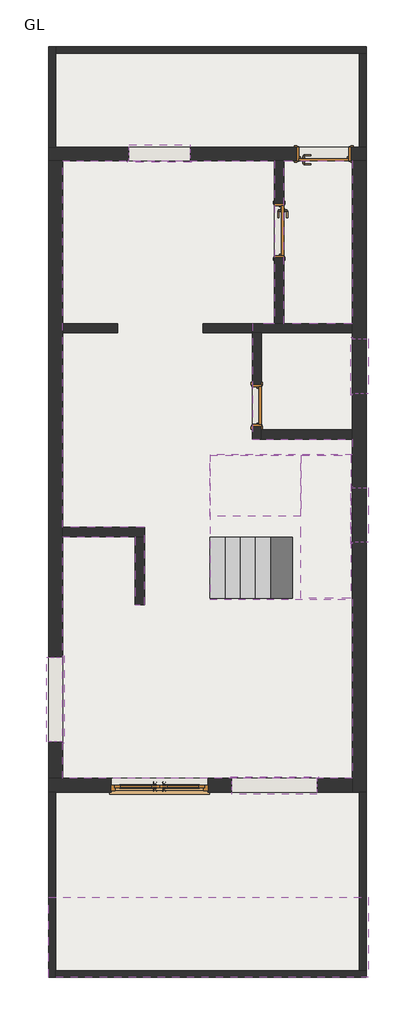
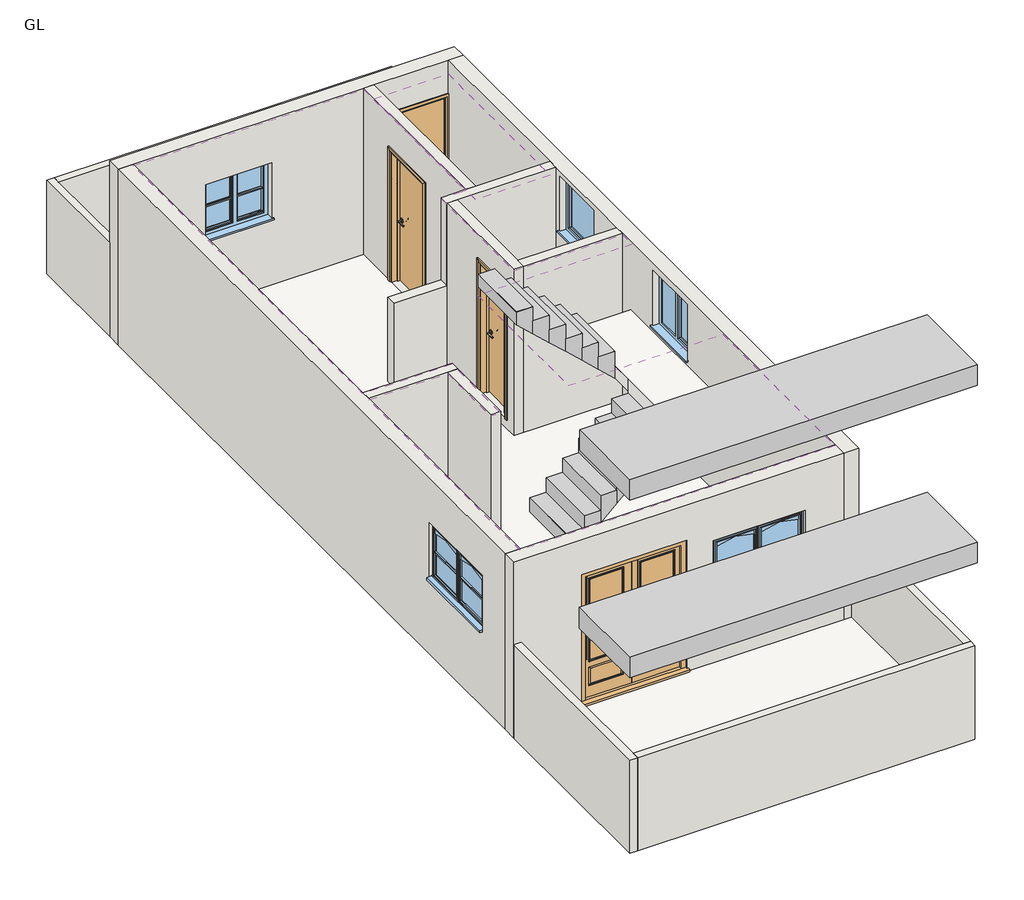
# One storey, incomplete: 18 walls, 6 slabs, 5 windows, 4 doors, 2 coverings, 2 stair flights, 1 furniture element.
"""IFC4 building model written with IfcOpenShell, lengths in millimetres."""

from ifc_helpers import new_model, si_unit, frame, origin, origin_with_axes, place, context, project, spatial, polyline, outline, extrude, faceted_brep, transform, mapped, element, save
from components import doors_extdbl_w_glazing_bars_2_f0b4ebcb, doors_extdbl_w_glazing_bars_2_fbc7e696, doors_intsgl_1_0_7m_00cad461, doors_intsgl_1_0_9m_9bbf83a0, doors_intsgl_1_0_9m_7aac3a70, casework_2_casework_2_475e0740, windows_dbl_swept_head_1_m_37dff1ae, windows_dbl_swept_head_1_4_m_8667dff2, windows_dbl_variable_casement_3235f540, windows_sgl_plain_0_9_m_ad1c2cf7

model = new_model("IFC4")

# Units and contexts
model_context = context("Model", 3, world=origin())
ifc_project = project(units=[si_unit("LENGTHUNIT", "METRE", prefix="MILLI")], contexts=[model_context])

# Site, building, storey
site = spatial("IfcSite", under=ifc_project)
building = spatial("IfcBuilding", under=site)
storey = spatial("IfcBuildingStorey", under=building, Name="GL", Elevation=0.0)

# Coverings
placement = place(None, origin())
element("IfcCovering", 1, ObjectType="Plain", at=placement, inside=storey, context=model_context, shape_type="SweptSolid", body=[
    extrude(outline(polyline([(-17484.6794706, 12010.5758404), (-16354.2794706, 12010.5758404), (-16354.2794706, 9327.0908033), (-17484.6794706, 9327.0908033), (-17484.6794706, 12010.5758404)])), frame((0.0, 0.0, 2600.0), z_axis=(0.0, 0.0, 1.0), x_axis=(1.0, 0.0, 0.0)), (0.0, 0.0, 1.0), 57.0),
])
element("IfcCovering", 2, ObjectType="Plain", at=placement, inside=storey, context=model_context, shape_type="SweptSolid", body=[
    extrude(outline(polyline([(-21137.0794706, 12010.5758404), (-17637.0794706, 12010.5758404), (-17637.0794706, 9327.0908033), (-18006.6794706, 9327.0908033), (-18006.6794706, 7422.2908033), (-16354.2794706, 7422.2908033), (-16354.2794706, 7168.7350753), (-18701.8794706, 7168.7350753), (-18701.8794706, 4785.9166056), (-16354.2794706, 4785.9166056), (-16354.2794706, 1829.2258404), (-21137.0794706, 1829.2258404), (-21137.0794706, 5814.1913528), (-19937.0794706, 5814.1913528), (-19937.0794706, 4690.3913528), (-19784.6794706, 4690.3913528), (-19784.6794706, 5966.5913528), (-21137.0794706, 5966.5913528), (-21137.0794706, 12010.5758404)])), frame((0.0, 0.0, 2800.0), z_axis=(0.0, 0.0, 1.0), x_axis=(1.0, 0.0, 0.0)), (0.0, 0.0, 1.0), 57.0),
])

# Doors
doors_extdbl_w_glazing_bars_2_shape = doors_extdbl_w_glazing_bars_2_f0b4ebcb(model_context)
doors_extdbl_w_glazing_bars_2_2_shape = doors_extdbl_w_glazing_bars_2_fbc7e696(model_context)
element("IfcDoor", 3, ObjectType="Doors_ExtDbl_w-Glazing_Bars_2", at=placement, inside=storey, context=model_context, shape_type="MappedRepresentation", body=[
    mapped(doors_extdbl_w_glazing_bars_2_shape, transform((-19537.0794706, 1714.9258404, 150.0), x_axis=(-1.0, 0.0, 0.0), y_axis=(0.0, -1.0, 0.0), z_axis=(0.0, 0.0, 1.0))),
    mapped(doors_extdbl_w_glazing_bars_2_2_shape, transform((-19537.0794706, 1714.9258404, 150.0), x_axis=(-1.0, 0.0, 0.0), y_axis=(0.0, -1.0, 0.0), z_axis=(0.0, 0.0, 1.0))),
])
doors_intsgl_1_0_7m_shape = doors_intsgl_1_0_7m_00cad461(model_context)
element("IfcDoor", 4, ObjectType="Doors_IntSgl_1 : 0.7M", at=placement, inside=storey, context=model_context, shape_type="MappedRepresentation", body=[
    mapped(doors_intsgl_1_0_7m_shape, transform((-17930.4794706, 7974.6908033, 300.0), x_axis=(0.0, -1.0, 0.0), y_axis=(1.0, 0.0, 0.0), z_axis=(0.0, 0.0, 1.0))),
])
doors_intsgl_1_0_9m_shape = doors_intsgl_1_0_9m_9bbf83a0(model_context)
element("IfcDoor", 5, ObjectType="Doors_IntSgl_1 : 0.9M", at=placement, inside=storey, context=model_context, shape_type="MappedRepresentation", body=[
    mapped(doors_intsgl_1_0_9m_shape, transform((-16824.2794706, 12124.8758404, 150.0), x_axis=(1.0, 0.0, 0.0), y_axis=(0.0, 1.0, 0.0), z_axis=(0.0, 0.0, 1.0))),
])
doors_intsgl_1_0_9m_2_shape = doors_intsgl_1_0_9m_7aac3a70(model_context)
element("IfcDoor", 6, ObjectType="Doors_IntSgl_1 : 0.9M", at=placement, inside=storey, context=model_context, shape_type="MappedRepresentation", body=[
    mapped(doors_intsgl_1_0_9m_2_shape, transform((-17560.8794706, 10860.5758404, 150.0), x_axis=(0.0, -1.0, 0.0), y_axis=(1.0, 0.0, 0.0), z_axis=(0.0, 0.0, 1.0))),
])

# Furniture
casework_2_casework_2_shape = casework_2_casework_2_475e0740(model_context)
element("IfcFurniture", 7, ObjectType="Casework 2 : Casework 2", at=placement, inside=storey, context=model_context, shape_type="MappedRepresentation", body=[
    mapped(casework_2_casework_2_shape, transform((0.0, 0.0, 0.0), x_axis=(1.0, 0.0, 0.0), y_axis=(0.0, 1.0, 0.0), z_axis=(0.0, 0.0, 1.0))),
])

# Slabs
element("IfcSlab", 8, at=placement, inside=storey, context=model_context, shape_type="SweptSolid", body=[
    extrude(outline(polyline([(-16239.9794706, 13782.0258404), (-16239.9794706, 12239.1758404), (-21251.3794706, 12239.1758404), (-21251.3794706, 13782.0258404), (-16239.9794706, 13782.0258404)])), origin_with_axes(), (0.0, 0.0, 1.0), 150.0),
])
element("IfcSlab", 9, ObjectType="200mm_Thickness", at=placement, inside=storey, context=model_context, shape_type="SolidModel", body=[
    faceted_brep([(-17201.8794706, 5801.1258404, 1764.3846154), (-17201.8794706, 4801.1258404, 1764.3846154), (-16947.3985621, 4801.1258404, 1764.3846154), (-16381.8794706, 4801.1258404, 1764.3846154), (-16381.8794706, 7153.5258404, 1764.3846154), (-17201.8794706, 7153.5258404, 1764.3846154), (-17201.8794706, 6153.5258404, 1764.3846154), (-17201.8794706, 5801.1258404, 1564.3846154), (-17201.8794706, 5801.1258404, 1533.6153846), (-17201.8794706, 5801.1258404, 1329.4791614), (-17201.8794706, 4801.1258404, 1329.4791614), (-17201.8794706, 4801.1258404, 1533.6153846), (-16947.3985621, 4801.1258404, 1564.3846154), (-16381.8794706, 4801.1258404, 1564.3846154), (-16381.8794706, 7153.5258404, 1564.3846154), (-17201.8794706, 7153.5258404, 1564.3846154), (-17201.8794706, 6153.5258404, 1564.3846154), (-16947.3985621, 5801.1258404, 1564.3846154)], [[[0, 1, 2, 3, 4, 5, 6]], [[1, 0, 7, 8, 9, 10, 11]], [[1, 11, 10, 12, 13, 3, 2]], [[4, 3, 13, 14]], [[5, 4, 14, 15]], [[6, 5, 15, 16]], [[0, 6, 16, 7]], [[12, 17, 7, 16, 15, 14, 13]], [[17, 12, 10, 9]], [[7, 17, 9, 8]]]),
    extrude(outline(polyline([(-17201.8794706, 5801.1258404), (-17201.8794706, 6153.5258404), (-17201.8794706, 7153.5258404), (-16381.8794706, 7153.5258404), (-16381.8794706, 4801.1258404), (-17201.8794706, 4801.1258404), (-17201.8794706, 5801.1258404)])), frame((0.0, 0.0, 1764.3846154), z_axis=(0.0, 0.0, 1.0), x_axis=(1.0, 0.0, 0.0)), (0.0, 0.0, 1.0), 1.0),
])
element("IfcSlab", 10, ObjectType="MAIN FLOOR", at=placement, inside=storey, context=model_context, shape_type="SweptSolid", body=[
    extrude(outline(polyline([(-16354.2794706, 1829.2258404), (-21137.0794706, 1829.2258404), (-21137.0794706, 9174.6908033), (-20231.3794706, 9174.6908033), (-20231.3794706, 9327.0908033), (-21137.0794706, 9327.0908033), (-21137.0794706, 12010.5758404), (-17637.0794706, 12010.5758404), (-17637.0794706, 9327.0908033), (-18819.9794706, 9327.0908033), (-18819.9794706, 9174.6908033), (-18006.6794706, 9174.6908033), (-18006.6794706, 7422.2908033), (-16354.2794706, 7422.2908033), (-16354.2794706, 1829.2258404)])), origin_with_axes(), (0.0, 0.0, 1.0), 150.0),
])
element("IfcSlab", 11, ObjectType="PARKING FLOOR", at=placement, inside=storey, context=model_context, shape_type="SweptSolid", body=[
    extrude(outline(polyline([(-16239.9794706, 1600.6258404), (-16239.9794706, -1339.3741596), (-21251.3794706, -1339.3741596), (-21251.3794706, 1600.6258404), (-16239.9794706, 1600.6258404)])), origin_with_axes(), (0.0, 0.0, 1.0), 150.0),
])
element("IfcSlab", 12, ObjectType="TOILET FLOOR", at=placement, inside=storey, context=model_context, shape_type="SweptSolid", body=[
    extrude(outline(polyline([(-17854.2794706, 7574.6908033), (-17854.2794706, 9174.6908033), (-16354.2794706, 9174.6908033), (-16354.2794706, 7574.6908033), (-17854.2794706, 7574.6908033)])), origin_with_axes(), (0.0, 0.0, 1.0), 300.0),
])
element("IfcSlab", 13, ObjectType="UTILITY FLOOR", at=placement, inside=storey, context=model_context, shape_type="SweptSolid", body=[
    extrude(outline(polyline([(-17484.6794706, 9327.0908033), (-17484.6794706, 12010.5758404), (-16354.2794706, 12010.5758404), (-16354.2794706, 9327.0908033), (-17484.6794706, 9327.0908033)])), origin_with_axes(), (0.0, 0.0, 1.0), 150.0),
])

# Stair flights
element("IfcStairFlight", 14, ObjectType="1mm_Tread-150mm_Depth", at=placement, inside=storey, context=model_context, shape_type="SolidModel", body=[
    faceted_brep([(-18451.8794706, 5801.1258404, 379.7692308), (-18701.8794706, 5801.1258404, 379.7692308), (-18701.8794706, 4801.1258404, 379.7692308), (-18451.8794706, 4801.1258404, 379.7692308), (-18451.8794706, 5801.1258404, 175.6330075), (-18479.6485621, 5801.1258404, 150.0), (-18701.8794706, 5801.1258404, 150.0), (-18701.8794706, 4801.1258404, 150.0), (-18479.6485621, 4801.1258404, 150.0), (-18451.8794706, 4801.1258404, 175.6330075), (-18201.8794706, 5801.1258404, 610.5384615), (-18451.8794706, 5801.1258404, 610.5384615), (-18451.8794706, 4801.1258404, 610.5384615), (-18201.8794706, 4801.1258404, 610.5384615), (-18201.8794706, 5801.1258404, 406.4022383), (-18201.8794706, 4801.1258404, 406.4022383), (-17951.8794706, 5801.1258404, 841.3076923), (-18201.8794706, 5801.1258404, 841.3076923), (-18201.8794706, 4801.1258404, 841.3076923), (-17951.8794706, 4801.1258404, 841.3076923), (-17951.8794706, 5801.1258404, 637.1714691), (-17951.8794706, 4801.1258404, 637.1714691), (-17701.8794706, 5801.1258404, 1072.0769231), (-17951.8794706, 5801.1258404, 1072.0769231), (-17951.8794706, 4801.1258404, 1072.0769231), (-17701.8794706, 4801.1258404, 1072.0769231), (-17701.8794706, 5801.1258404, 867.9406999), (-17701.8794706, 4801.1258404, 867.9406999), (-17451.8794706, 5801.1258404, 1302.8461538), (-17701.8794706, 5801.1258404, 1302.8461538), (-17701.8794706, 4801.1258404, 1302.8461538), (-17451.8794706, 4801.1258404, 1302.8461538), (-17451.8794706, 5801.1258404, 1098.7099306), (-17451.8794706, 4801.1258404, 1098.7099306), (-17201.8794706, 5801.1258404, 1533.6153846), (-17451.8794706, 5801.1258404, 1533.6153846), (-17451.8794706, 4801.1258404, 1533.6153846), (-17201.8794706, 4801.1258404, 1533.6153846), (-17201.8794706, 5801.1258404, 1329.4791614), (-17201.8794706, 4801.1258404, 1329.4791614)], [[[0, 1, 2, 3]], [[1, 0, 4, 5, 6]], [[2, 1, 6, 7]], [[3, 2, 7, 8, 9]], [[10, 11, 12, 13]], [[11, 10, 14, 4, 0]], [[0, 3, 12, 11]], [[13, 12, 3, 9, 15]], [[16, 17, 18, 19]], [[17, 16, 20, 14, 10]], [[10, 13, 18, 17]], [[19, 18, 13, 15, 21]], [[22, 23, 24, 25]], [[23, 22, 26, 20, 16]], [[16, 19, 24, 23]], [[25, 24, 19, 21, 27]], [[28, 29, 30, 31]], [[29, 28, 32, 26, 22]], [[22, 25, 30, 29]], [[31, 30, 25, 27, 33]], [[34, 35, 36, 37]], [[35, 34, 38, 32, 28]], [[28, 31, 36, 35]], [[37, 36, 31, 33, 39]], [[34, 37, 39, 38]], [[7, 6, 5, 8]], [[8, 5, 4, 14, 20, 26, 32, 38, 39, 33, 27, 21, 15, 9]]]),
    extrude(outline(polyline([(-18451.8794706, 5801.1258404), (-18451.8794706, 4801.1258404), (-18701.8794706, 4801.1258404), (-18701.8794706, 5801.1258404), (-18451.8794706, 5801.1258404)])), frame((0.0, 0.0, 379.7692308), z_axis=(0.0, 0.0, 1.0), x_axis=(1.0, 0.0, 0.0)), (0.0, 0.0, 1.0), 1.0),
    extrude(outline(polyline([(-18201.8794706, 5801.1258404), (-18201.8794706, 4801.1258404), (-18451.8794706, 4801.1258404), (-18451.8794706, 5801.1258404), (-18201.8794706, 5801.1258404)])), frame((0.0, 0.0, 610.5384615), z_axis=(0.0, 0.0, 1.0), x_axis=(1.0, 0.0, 0.0)), (0.0, 0.0, 1.0), 1.0),
    extrude(outline(polyline([(-17951.8794706, 5801.1258404), (-17951.8794706, 4801.1258404), (-18201.8794706, 4801.1258404), (-18201.8794706, 5801.1258404), (-17951.8794706, 5801.1258404)])), frame((0.0, 0.0, 841.3076923), z_axis=(0.0, 0.0, 1.0), x_axis=(1.0, 0.0, 0.0)), (0.0, 0.0, 1.0), 1.0),
    extrude(outline(polyline([(-17701.8794706, 5801.1258404), (-17701.8794706, 4801.1258404), (-17951.8794706, 4801.1258404), (-17951.8794706, 5801.1258404), (-17701.8794706, 5801.1258404)])), frame((0.0, 0.0, 1072.0769231), z_axis=(0.0, 0.0, 1.0), x_axis=(1.0, 0.0, 0.0)), (0.0, 0.0, 1.0), 1.0),
    extrude(outline(polyline([(-17451.8794706, 5801.1258404), (-17451.8794706, 4801.1258404), (-17701.8794706, 4801.1258404), (-17701.8794706, 5801.1258404), (-17451.8794706, 5801.1258404)])), frame((0.0, 0.0, 1302.8461538), z_axis=(0.0, 0.0, 1.0), x_axis=(1.0, 0.0, 0.0)), (0.0, 0.0, 1.0), 1.0),
    extrude(outline(polyline([(-17201.8794706, 5801.1258404), (-17201.8794706, 4801.1258404), (-17451.8794706, 4801.1258404), (-17451.8794706, 5801.1258404), (-17201.8794706, 5801.1258404)])), frame((0.0, 0.0, 1533.6153846), z_axis=(0.0, 0.0, 1.0), x_axis=(1.0, 0.0, 0.0)), (0.0, 0.0, 1.0), 1.0),
])
element("IfcStairFlight", 15, ObjectType="1mm_Tread-150mm_Depth", at=placement, inside=storey, context=model_context, shape_type="SolidModel", body=[
    faceted_brep([(-17201.8794706, 6153.5258404, 1995.1538462), (-17201.8794706, 7153.5258404, 1995.1538462), (-17206.3603791, 7153.5258404, 1995.1538462), (-17451.8794706, 7153.5258404, 1995.1538462), (-17451.8794706, 6153.5258404, 1995.1538462), (-17206.3603791, 6153.5258404, 1995.1538462), (-17451.8794706, 6153.5258404, 1791.0176229), (-17206.3603791, 6153.5258404, 1564.3846154), (-17201.8794706, 6153.5258404, 1564.3846154), (-17201.8794706, 7153.5258404, 1564.3846154), (-17201.8794706, 7153.5258404, 1764.3846154), (-17206.3603791, 7153.5258404, 1564.3846154), (-17451.8794706, 7153.5258404, 1791.0176229), (-17701.8794706, 6153.5258404, 2225.9230769), (-17451.8794706, 6153.5258404, 2225.9230769), (-17451.8794706, 7153.5258404, 2225.9230769), (-17701.8794706, 7153.5258404, 2225.9230769), (-17701.8794706, 6153.5258404, 2021.7868537), (-17701.8794706, 7153.5258404, 2021.7868537), (-17951.8794706, 6153.5258404, 2456.6923077), (-17701.8794706, 6153.5258404, 2456.6923077), (-17701.8794706, 7153.5258404, 2456.6923077), (-17951.8794706, 7153.5258404, 2456.6923077), (-17951.8794706, 6153.5258404, 2252.5560845), (-17951.8794706, 7153.5258404, 2252.5560845), (-18201.8794706, 6153.5258404, 2687.4615385), (-17951.8794706, 6153.5258404, 2687.4615385), (-17951.8794706, 7153.5258404, 2687.4615385), (-18201.8794706, 7153.5258404, 2687.4615385), (-18201.8794706, 6153.5258404, 2483.3253152), (-18201.8794706, 7153.5258404, 2483.3253152), (-18451.8794706, 6153.5258404, 2918.2307692), (-18201.8794706, 6153.5258404, 2918.2307692), (-18201.8794706, 7153.5258404, 2918.2307692), (-18451.8794706, 7153.5258404, 2918.2307692), (-18451.8794706, 6153.5258404, 2714.094546), (-18451.8794706, 7153.5258404, 2714.094546), (-18701.8794706, 6153.5258404, 3149.0), (-18451.8794706, 6153.5258404, 3149.0), (-18451.8794706, 7153.5258404, 3149.0), (-18701.8794706, 7153.5258404, 3149.0), (-18701.8794706, 6153.5258404, 2944.8637768), (-18701.8794706, 7153.5258404, 2944.8637768)], [[[0, 1, 2, 3, 4, 5]], [[4, 6, 7, 8, 0, 5]], [[1, 0, 8, 9, 10]], [[1, 10, 9, 11, 12, 3, 2]], [[13, 14, 15, 16]], [[14, 13, 17, 6, 4]], [[15, 14, 4, 3]], [[16, 15, 3, 12, 18]], [[19, 20, 21, 22]], [[20, 19, 23, 17, 13]], [[21, 20, 13, 16]], [[22, 21, 16, 18, 24]], [[25, 26, 27, 28]], [[26, 25, 29, 23, 19]], [[27, 26, 19, 22]], [[28, 27, 22, 24, 30]], [[31, 32, 33, 34]], [[32, 31, 35, 29, 25]], [[33, 32, 25, 28]], [[34, 33, 28, 30, 36]], [[37, 38, 39, 40]], [[38, 37, 41, 35, 31]], [[39, 38, 31, 34]], [[40, 39, 34, 36, 42]], [[37, 40, 42, 41]], [[11, 7, 6, 17, 23, 29, 35, 41, 42, 36, 30, 24, 18, 12]], [[7, 11, 9, 8]]]),
    extrude(outline(polyline([(-17451.8794706, 6153.5258404), (-17451.8794706, 7153.5258404), (-17201.8794706, 7153.5258404), (-17201.8794706, 6153.5258404), (-17451.8794706, 6153.5258404)])), frame((0.0, 0.0, 1995.1538462), z_axis=(0.0, 0.0, 1.0), x_axis=(1.0, 0.0, 0.0)), (0.0, 0.0, 1.0), 1.0),
    extrude(outline(polyline([(-17701.8794706, 6153.5258404), (-17701.8794706, 7153.5258404), (-17451.8794706, 7153.5258404), (-17451.8794706, 6153.5258404), (-17701.8794706, 6153.5258404)])), frame((0.0, 0.0, 2225.9230769), z_axis=(0.0, 0.0, 1.0), x_axis=(1.0, 0.0, 0.0)), (0.0, 0.0, 1.0), 1.0),
    extrude(outline(polyline([(-17951.8794706, 6153.5258404), (-17951.8794706, 7153.5258404), (-17701.8794706, 7153.5258404), (-17701.8794706, 6153.5258404), (-17951.8794706, 6153.5258404)])), frame((0.0, 0.0, 2456.6923077), z_axis=(0.0, 0.0, 1.0), x_axis=(1.0, 0.0, 0.0)), (0.0, 0.0, 1.0), 1.0),
    extrude(outline(polyline([(-18201.8794706, 6153.5258404), (-18201.8794706, 7153.5258404), (-17951.8794706, 7153.5258404), (-17951.8794706, 6153.5258404), (-18201.8794706, 6153.5258404)])), frame((0.0, 0.0, 2687.4615385), z_axis=(0.0, 0.0, 1.0), x_axis=(1.0, 0.0, 0.0)), (0.0, 0.0, 1.0), 1.0),
    extrude(outline(polyline([(-18451.8794706, 6153.5258404), (-18451.8794706, 7153.5258404), (-18201.8794706, 7153.5258404), (-18201.8794706, 6153.5258404), (-18451.8794706, 6153.5258404)])), frame((0.0, 0.0, 2918.2307692), z_axis=(0.0, 0.0, 1.0), x_axis=(1.0, 0.0, 0.0)), (0.0, 0.0, 1.0), 1.0),
    extrude(outline(polyline([(-18701.8794706, 6153.5258404), (-18701.8794706, 7153.5258404), (-18451.8794706, 7153.5258404), (-18451.8794706, 6153.5258404), (-18701.8794706, 6153.5258404)])), frame((0.0, 0.0, 3149.0), z_axis=(0.0, 0.0, 1.0), x_axis=(1.0, 0.0, 0.0)), (0.0, 0.0, 1.0), 1.0),
])

# Walls
element("IfcWall", 16, at=placement, inside=storey, context=model_context, shape_type="Brep", body=[
    faceted_brep([(-16354.2794706, 9327.0908033, 0.0), (-17484.6794706, 9327.0908033, 0.0), (-17637.0794706, 9327.0908033, 0.0), (-18009.9794706, 9327.0908033, 0.0), (-18009.9794706, 9327.0908033, 1500.0), (-18009.9794706, 9327.0908033, 2820.0), (-17637.0794706, 9327.0908033, 2820.0), (-17484.6794706, 9327.0908033, 2820.0), (-16354.2794706, 9327.0908033, 2820.0), (-16354.2794706, 9174.6908033, 0.0), (-16354.2794706, 9174.6908033, 2820.0), (-17854.2794706, 9174.6908033, 2820.0), (-18006.6794706, 9174.6908033, 2820.0), (-18009.9794706, 9174.6908033, 2820.0), (-18009.9794706, 9174.6908033, 1500.0), (-18009.9794706, 9174.6908033, 0.0), (-18006.6794706, 9174.6908033, 0.0), (-17854.2794706, 9174.6908033, 0.0)], [[[0, 1, 2, 3, 4, 5, 6, 7, 8]], [[9, 10, 11, 12, 13, 14, 15, 16, 17]], [[3, 2, 1, 0, 9, 17, 16, 15]], [[5, 4, 3, 15, 14, 13]], [[8, 7, 6, 5, 13, 12, 11, 10]], [[0, 8, 10, 9]]]),
])
element("IfcWall", 17, at=placement, inside=storey, context=model_context, shape_type="SweptSolid", body=[
    extrude(outline(polyline([(9327.0908033, 0.0), (9327.0908033, 2820.0), (12010.5758404, 2820.0), (12010.5758404, 0.0), (9327.0908033, 0.0)]), holes=[polyline([(10410.5758404, 150.0), (11310.5758404, 150.0), (11310.5758404, 2260.0), (10410.5758404, 2260.0), (10410.5758404, 150.0)])]), frame((-17637.0794706, 0.0, 0.0), z_axis=(1.0, 0.0, 0.0), x_axis=(0.0, 1.0, 0.0)), (0.0, 0.0, 1.0), 152.4),
])
element("IfcWall", 18, at=placement, inside=storey, context=model_context, shape_type="Brep", body=[
    faceted_brep([(-18006.6794706, 9174.6908033, 0.0), (-18006.6794706, 7422.2908033, 0.0), (-18006.6794706, 7422.2908033, 2820.0), (-18006.6794706, 9174.6908033, 2820.0), (-18006.6794706, 7624.6908033, 300.0), (-18006.6794706, 8324.6908033, 300.0), (-18006.6794706, 8324.6908033, 2410.0), (-18006.6794706, 7624.6908033, 2410.0), (-17854.2794706, 9174.6908033, 0.0), (-17854.2794706, 9174.6908033, 2820.0), (-17854.2794706, 7574.6908033, 2820.0), (-17854.2794706, 7422.2908033, 2820.0), (-17854.2794706, 7422.2908033, 0.0), (-17854.2794706, 7574.6908033, 0.0), (-17854.2794706, 7624.6908033, 300.0), (-17854.2794706, 7624.6908033, 2410.0), (-17854.2794706, 8324.6908033, 2410.0), (-17854.2794706, 8324.6908033, 300.0)], [[[0, 1, 2, 3], [4, 5, 6, 7]], [[8, 9, 10, 11, 12, 13], [14, 15, 16, 17]], [[1, 0, 8, 13, 12]], [[3, 2, 11, 10, 9]], [[0, 3, 9, 8]], [[2, 1, 12, 11]], [[15, 14, 4, 7]], [[16, 15, 7, 6]], [[17, 16, 6, 5]], [[14, 17, 5, 4]]]),
])
element("IfcWall", 19, at=placement, inside=storey, context=model_context, shape_type="SweptSolid", body=[
    extrude(outline(polyline([(-16354.2794706, 7422.2908033), (-17854.2794706, 7422.2908033), (-17854.2794706, 7574.6908033), (-16354.2794706, 7574.6908033), (-16354.2794706, 7422.2908033)])), origin_with_axes(), (0.0, 0.0, 1.0), 2820.0),
])
element("IfcWall", 20, at=placement, inside=storey, context=model_context, shape_type="SweptSolid", body=[
    extrude(outline(polyline([(-21137.0794706, 9327.0908033), (-20231.3794706, 9327.0908033), (-20231.3794706, 9174.6908033), (-21137.0794706, 9174.6908033), (-21137.0794706, 9327.0908033)])), origin_with_axes(), (0.0, 0.0, 1.0), 1500.0),
])
element("IfcWall", 21, at=placement, inside=storey, context=model_context, shape_type="Brep", body=[
    faceted_brep([(-21137.0794706, 5814.1913528, 0.0), (-19937.0794706, 5814.1913528, 0.0), (-19784.6794706, 5814.1913528, 0.0), (-19784.6794706, 5814.1913528, 2820.0), (-19937.0794706, 5814.1913528, 2820.0), (-21137.0794706, 5814.1913528, 2820.0), (-21137.0794706, 5966.5913528, 0.0), (-21137.0794706, 5966.5913528, 2820.0), (-19784.6794706, 5966.5913528, 2820.0), (-19784.6794706, 5966.5913528, 0.0)], [[[0, 1, 2, 3, 4, 5]], [[6, 7, 8, 9]], [[2, 1, 0, 6, 9]], [[5, 4, 3, 8, 7]], [[0, 5, 7, 6]], [[3, 2, 9, 8]]]),
])
element("IfcWall", 22, at=placement, inside=storey, context=model_context, shape_type="SweptSolid", body=[
    extrude(outline(polyline([(-19937.0794706, 4690.3913528), (-19937.0794706, 5814.1913528), (-19784.6794706, 5814.1913528), (-19784.6794706, 4690.3913528), (-19937.0794706, 4690.3913528)])), origin_with_axes(), (0.0, 0.0, 1.0), 2820.0),
])
element("IfcWall", 23, at=placement, inside=storey, context=model_context, shape_type="SweptSolid", body=[
    extrude(outline(polyline([(-18819.9794706, 9327.0908033), (-18009.9794706, 9327.0908033), (-18009.9794706, 9174.6908033), (-18819.9794706, 9174.6908033), (-18819.9794706, 9327.0908033)])), origin_with_axes(), (0.0, 0.0, 1.0), 1500.0),
])
element("IfcWall", 24, ObjectType="EX WALL", at=placement, inside=storey, context=model_context, shape_type="Brep", body=[
    faceted_brep([(-21365.6794706, 12010.5758404, 2820.0), (-21365.6794706, 12010.5758404, 0.0), (-21137.0794706, 12010.5758404, 0.0), (-17637.0794706, 12010.5758404, 0.0), (-17484.6794706, 12010.5758404, 0.0), (-16354.2794706, 12010.5758404, 0.0), (-16125.6794706, 12010.5758404, 0.0), (-16125.6794706, 12010.5758404, 2820.0), (-16354.2794706, 12010.5758404, 2820.0), (-17484.6794706, 12010.5758404, 2820.0), (-17637.0794706, 12010.5758404, 2820.0), (-21137.0794706, 12010.5758404, 2820.0), (-16374.2794706, 12010.5758404, 150.0), (-17274.2794706, 12010.5758404, 150.0), (-17274.2794706, 12010.5758404, 2260.0), (-16374.2794706, 12010.5758404, 2260.0), (-20037.0794706, 12010.5758404, 2110.0), (-19037.0794706, 12010.5758404, 2110.0), (-19037.0794706, 12010.5758404, 1200.0), (-20037.0794706, 12010.5758404, 1200.0), (-21365.6794706, 12239.1758404, 0.0), (-21365.6794706, 12239.1758404, 1500.0), (-21365.6794706, 12239.1758404, 2820.0), (-16125.6794706, 12239.1758404, 2820.0), (-16125.6794706, 12239.1758404, 1500.0), (-16125.6794706, 12239.1758404, 0.0), (-16239.9794706, 12239.1758404, 0.0), (-21251.3794706, 12239.1758404, 0.0), (-16374.2794706, 12239.1758404, 150.0), (-16374.2794706, 12239.1758404, 2260.0), (-17274.2794706, 12239.1758404, 2260.0), (-17274.2794706, 12239.1758404, 150.0), (-20037.0794706, 12239.1758404, 2110.0), (-20037.0794706, 12239.1758404, 1200.0), (-19037.0794706, 12239.1758404, 1200.0), (-19037.0794706, 12239.1758404, 2110.0)], [[[0, 1, 2, 3, 4, 5, 6, 7, 8, 9, 10, 11], [12, 13, 14, 15], [16, 17, 18, 19]], [[20, 21, 22, 23, 24, 25, 26, 27], [28, 29, 30, 31], [32, 33, 34, 35]], [[6, 5, 4, 3, 2, 1, 20, 27, 26, 25]], [[0, 11, 10, 9, 8, 7, 23, 22]], [[0, 22, 21, 20, 1]], [[6, 25, 24, 23, 7]], [[29, 28, 12, 15]], [[30, 29, 15, 14]], [[31, 30, 14, 13]], [[28, 31, 13, 12]], [[33, 32, 16, 19]], [[34, 33, 19, 18]], [[35, 34, 18, 17]], [[32, 35, 17, 16]]]),
])
element("IfcWall", 25, ObjectType="EX WALL", at=placement, inside=storey, context=model_context, shape_type="Brep", body=[
    faceted_brep([(-16354.2794706, 12010.5758404, 2820.0), (-16354.2794706, 12010.5758404, 0.0), (-16354.2794706, 9327.0908033, 0.0), (-16354.2794706, 9174.6908033, 0.0), (-16354.2794706, 7574.6908033, 0.0), (-16354.2794706, 7422.2908033, 0.0), (-16354.2794706, 1829.2258404, 0.0), (-16354.2794706, 1600.6258404, 0.0), (-16354.2794706, 1600.6258404, 2820.0), (-16354.2794706, 1829.2258404, 2820.0), (-16354.2794706, 7422.2908033, 2820.0), (-16354.2794706, 7574.6908033, 2820.0), (-16354.2794706, 9174.6908033, 2820.0), (-16354.2794706, 9327.0908033, 2820.0), (-16354.2794706, 9074.6908033, 2738.8), (-16354.2794706, 8174.6908033, 2738.8), (-16354.2794706, 8174.6908033, 1828.8), (-16354.2794706, 9074.6908033, 1828.8), (-16354.2794706, 6622.2908033, 2710.0), (-16354.2794706, 5722.2908033, 2710.0), (-16354.2794706, 5722.2908033, 1800.0), (-16354.2794706, 6622.2908033, 1800.0), (-16125.6794706, 12010.5758404, 0.0), (-16125.6794706, 12010.5758404, 2820.0), (-16125.6794706, 1600.6258404, 2820.0), (-16125.6794706, 1600.6258404, 1500.0), (-16125.6794706, 1600.6258404, 0.0), (-16125.6794706, 9074.6908033, 2738.8), (-16125.6794706, 9074.6908033, 1828.8), (-16125.6794706, 8174.6908033, 1828.8), (-16125.6794706, 8174.6908033, 2738.8), (-16125.6794706, 6622.2908033, 2710.0), (-16125.6794706, 6622.2908033, 1800.0), (-16125.6794706, 5722.2908033, 1800.0), (-16125.6794706, 5722.2908033, 2710.0), (-16239.9794706, 1600.6258404, 0.0)], [[[0, 1, 2, 3, 4, 5, 6, 7, 8, 9, 10, 11, 12, 13], [14, 15, 16, 17], [18, 19, 20, 21]], [[22, 23, 24, 25, 26], [27, 28, 29, 30], [31, 32, 33, 34]], [[7, 6, 5, 4, 3, 2, 1, 22, 26, 35]], [[0, 13, 12, 11, 10, 9, 8, 24, 23]], [[0, 23, 22, 1]], [[7, 35, 26, 25, 24, 8]], [[28, 27, 14, 17]], [[29, 28, 17, 16]], [[30, 29, 16, 15]], [[27, 30, 15, 14]], [[32, 31, 18, 21]], [[33, 32, 21, 20]], [[34, 33, 20, 19]], [[31, 34, 19, 18]]]),
])
element("IfcWall", 26, ObjectType="EX WALL", at=placement, inside=storey, context=model_context, shape_type="Brep", body=[
    faceted_brep([(-16354.2794706, 1829.2258404, 0.0), (-21137.0794706, 1829.2258404, 0.0), (-21365.6794706, 1829.2258404, 0.0), (-21365.6794706, 1829.2258404, 2820.0), (-21137.0794706, 1829.2258404, 2820.0), (-16354.2794706, 1829.2258404, 2820.0), (-18737.0794706, 1829.2258404, 150.0), (-18737.0794706, 1829.2258404, 2260.0), (-20337.0794706, 1829.2258404, 2260.0), (-20337.0794706, 1829.2258404, 150.0), (-16937.0794706, 1829.2258404, 1200.0), (-16937.0794706, 1829.2258404, 2110.0), (-18337.0794706, 1829.2258404, 2110.0), (-18337.0794706, 1829.2258404, 1200.0), (-21365.6794706, 1600.6258404, 0.0), (-21251.3794706, 1600.6258404, 0.0), (-16354.2794706, 1600.6258404, 0.0), (-16354.2794706, 1600.6258404, 2820.0), (-21365.6794706, 1600.6258404, 2820.0), (-21365.6794706, 1600.6258404, 1500.0), (-18737.0794706, 1600.6258404, 2260.0), (-18737.0794706, 1600.6258404, 150.0), (-20337.0794706, 1600.6258404, 150.0), (-20337.0794706, 1600.6258404, 2260.0), (-16937.0794706, 1600.6258404, 2110.0), (-16937.0794706, 1600.6258404, 1200.0), (-18337.0794706, 1600.6258404, 1200.0), (-18337.0794706, 1600.6258404, 2110.0)], [[[0, 1, 2, 3, 4, 5], [6, 7, 8, 9], [10, 11, 12, 13]], [[14, 15, 16, 17, 18, 19], [20, 21, 22, 23], [24, 25, 26, 27]], [[2, 1, 0, 16, 15, 14]], [[5, 4, 3, 18, 17]], [[2, 14, 19, 18, 3]], [[5, 17, 16, 0]], [[6, 21, 20, 7]], [[7, 20, 23, 8]], [[8, 23, 22, 9]], [[21, 6, 9, 22]], [[25, 24, 11, 10]], [[26, 25, 10, 13]], [[27, 26, 13, 12]], [[24, 27, 12, 11]]]),
])
element("IfcWall", 27, ObjectType="EX WALL", at=placement, inside=storey, context=model_context, shape_type="Brep", body=[
    faceted_brep([(-21137.0794706, 1829.2258404, 2820.0), (-21137.0794706, 1829.2258404, 0.0), (-21137.0794706, 5814.1913528, 0.0), (-21137.0794706, 5966.5913528, 0.0), (-21137.0794706, 9174.6908033, 0.0), (-21137.0794706, 9327.0908033, 0.0), (-21137.0794706, 12010.5758404, 0.0), (-21137.0794706, 12010.5758404, 2820.0), (-21137.0794706, 5966.5913528, 2820.0), (-21137.0794706, 5814.1913528, 2820.0), (-21137.0794706, 2429.2258404, 2110.0), (-21137.0794706, 3829.2258404, 2110.0), (-21137.0794706, 3829.2258404, 1200.0), (-21137.0794706, 2429.2258404, 1200.0), (-21365.6794706, 1829.2258404, 0.0), (-21365.6794706, 1829.2258404, 2820.0), (-21365.6794706, 12010.5758404, 2820.0), (-21365.6794706, 12010.5758404, 0.0), (-21365.6794706, 2429.2258404, 2110.0), (-21365.6794706, 2429.2258404, 1200.0), (-21365.6794706, 3829.2258404, 1200.0), (-21365.6794706, 3829.2258404, 2110.0)], [[[0, 1, 2, 3, 4, 5, 6, 7, 8, 9], [10, 11, 12, 13]], [[14, 15, 16, 17], [18, 19, 20, 21]], [[6, 5, 4, 3, 2, 1, 14, 17]], [[0, 9, 8, 7, 16, 15]], [[0, 15, 14, 1]], [[19, 18, 10, 13]], [[20, 19, 13, 12]], [[21, 20, 12, 11]], [[18, 21, 11, 10]], [[7, 6, 17, 16]]]),
])
element("IfcWall", 28, ObjectType="OUT WALL", at=placement, inside=storey, context=model_context, shape_type="Brep", body=[
    faceted_brep([(-21251.3794706, 12239.1758404, 0.0), (-21251.3794706, 13782.0258404, 0.0), (-21251.3794706, 13896.3258404, 0.0), (-21251.3794706, 13896.3258404, 1500.0), (-21251.3794706, 13782.0258404, 1500.0), (-21251.3794706, 12239.1758404, 1500.0), (-21365.6794706, 12239.1758404, 0.0), (-21365.6794706, 12239.1758404, 1500.0), (-21365.6794706, 13896.3258404, 1500.0), (-21365.6794706, 13896.3258404, 0.0)], [[[0, 1, 2, 3, 4, 5]], [[6, 7, 8, 9]], [[2, 1, 0, 6, 9]], [[5, 4, 3, 8, 7]], [[0, 5, 7, 6]], [[3, 2, 9, 8]]]),
])
element("IfcWall", 29, ObjectType="OUT WALL", at=placement, inside=storey, context=model_context, shape_type="Brep", body=[
    faceted_brep([(-21251.3794706, 13782.0258404, 0.0), (-16239.9794706, 13782.0258404, 0.0), (-16125.6794706, 13782.0258404, 0.0), (-16125.6794706, 13782.0258404, 1500.0), (-16239.9794706, 13782.0258404, 1500.0), (-21251.3794706, 13782.0258404, 1500.0), (-21251.3794706, 13896.3258404, 0.0), (-21251.3794706, 13896.3258404, 1500.0), (-16125.6794706, 13896.3258404, 1500.0), (-16125.6794706, 13896.3258404, 0.0)], [[[0, 1, 2, 3, 4, 5]], [[6, 7, 8, 9]], [[2, 1, 0, 6, 9]], [[5, 4, 3, 8, 7]], [[0, 5, 7, 6]], [[3, 2, 9, 8]]]),
])
element("IfcWall", 30, ObjectType="OUT WALL", at=placement, inside=storey, context=model_context, shape_type="SweptSolid", body=[
    extrude(outline(polyline([(-16239.9794706, 12239.1758404), (-16239.9794706, 13782.0258404), (-16125.6794706, 13782.0258404), (-16125.6794706, 12239.1758404), (-16239.9794706, 12239.1758404)])), origin_with_axes(), (0.0, 0.0, 1.0), 1500.0),
])
element("IfcWall", 31, ObjectType="OUT WALL", at=placement, inside=storey, context=model_context, shape_type="Brep", body=[
    faceted_brep([(-21365.6794706, 1600.6258404, 0.0), (-21365.6794706, -1453.6741596, 0.0), (-21365.6794706, -1453.6741596, 1500.0), (-21365.6794706, 1600.6258404, 1500.0), (-21251.3794706, 1600.6258404, 0.0), (-21251.3794706, 1600.6258404, 1500.0), (-21251.3794706, -1339.3741596, 1500.0), (-21251.3794706, -1453.6741596, 1500.0), (-21251.3794706, -1453.6741596, 0.0), (-21251.3794706, -1339.3741596, 0.0)], [[[0, 1, 2, 3]], [[4, 5, 6, 7, 8, 9]], [[1, 0, 4, 9, 8]], [[3, 2, 7, 6, 5]], [[0, 3, 5, 4]], [[2, 1, 8, 7]]]),
])
element("IfcWall", 32, ObjectType="OUT WALL", at=placement, inside=storey, context=model_context, shape_type="Brep", body=[
    faceted_brep([(-21251.3794706, -1453.6741596, 0.0), (-16125.6794706, -1453.6741596, 0.0), (-16125.6794706, -1453.6741596, 1500.0), (-21251.3794706, -1453.6741596, 1500.0), (-21251.3794706, -1339.3741596, 0.0), (-21251.3794706, -1339.3741596, 1500.0), (-16239.9794706, -1339.3741596, 1500.0), (-16125.6794706, -1339.3741596, 1500.0), (-16125.6794706, -1339.3741596, 0.0), (-16239.9794706, -1339.3741596, 0.0)], [[[0, 1, 2, 3]], [[4, 5, 6, 7, 8, 9]], [[1, 0, 4, 9, 8]], [[3, 2, 7, 6, 5]], [[0, 3, 5, 4]], [[2, 1, 8, 7]]]),
])
element("IfcWall", 33, ObjectType="OUT WALL", at=placement, inside=storey, context=model_context, shape_type="SweptSolid", body=[
    extrude(outline(polyline([(-16239.9794706, -1339.3741596), (-16239.9794706, 1600.6258404), (-16125.6794706, 1600.6258404), (-16125.6794706, -1339.3741596), (-16239.9794706, -1339.3741596)])), origin_with_axes(), (0.0, 0.0, 1.0), 1500.0),
])

# Windows
windows_dbl_swept_head_1_m_shape = windows_dbl_swept_head_1_m_37dff1ae(model_context)
element("IfcWindow", 34, ObjectType="Windows_Dbl_Swept_Head : 1 M", at=placement, inside=storey, context=model_context, shape_type="MappedRepresentation", body=[
    mapped(windows_dbl_swept_head_1_m_shape, transform((-19252.0794706, 12116.4192726, 0.0), x_axis=(1.0, 0.0, 0.0), y_axis=(0.0, 1.0, 0.0), z_axis=(0.0, 0.0, 1.0))),
])
windows_dbl_swept_head_1_4_m_shape = windows_dbl_swept_head_1_4_m_8667dff2(model_context)
element("IfcWindow", 35, ObjectType="Windows_Dbl_Swept_Head : 1.4 M", at=placement, inside=storey, context=model_context, shape_type="MappedRepresentation", body=[
    mapped(windows_dbl_swept_head_1_4_m_shape, transform((-17922.0794706, 1723.3824083, 0.0), x_axis=(-1.0, 0.0, 0.0), y_axis=(0.0, -1.0, 0.0), z_axis=(0.0, 0.0, 1.0))),
])
element("IfcWindow", 36, ObjectType="Windows_Dbl_Swept_Head : 1.4 M", at=placement, inside=storey, context=model_context, shape_type="MappedRepresentation", body=[
    mapped(windows_dbl_swept_head_1_4_m_shape, transform((-21242.9229028, 3414.2258404, 0.0), x_axis=(0.0, 1.0, 0.0), y_axis=(-1.0, 0.0, 0.0), z_axis=(0.0, 0.0, 1.0))),
])
windows_dbl_variable_casement_shape = windows_dbl_variable_casement_3235f540(model_context)
element("IfcWindow", 37, ObjectType="Windows_Dbl_Variable_Casement", at=placement, inside=storey, context=model_context, shape_type="MappedRepresentation", body=[
    mapped(windows_dbl_variable_casement_shape, transform((-16248.4360384, 5887.2908033, 600.0), x_axis=(0.0, -1.0, 0.0), y_axis=(1.0, 0.0, 0.0), z_axis=(0.0, 0.0, 1.0))),
])
windows_sgl_plain_0_9_m_shape = windows_sgl_plain_0_9_m_ad1c2cf7(model_context)
element("IfcWindow", 38, ObjectType="Windows_Sgl_Plain : 0.9 M", at=placement, inside=storey, context=model_context, shape_type="MappedRepresentation", body=[
    mapped(windows_sgl_plain_0_9_m_shape, transform((-16248.4360384, 8624.6908033, 628.8), x_axis=(0.0, -1.0, 0.0), y_axis=(1.0, 0.0, 0.0), z_axis=(0.0, 0.0, 1.0))),
])

save(model, "model.ifc")

# Revit data of these elements
# Type "Plain"
#   Keynote = "K40"
#   built-in parameter 1002203 = 1 (stored number, unit not read)
#   built-in parameter 1002202 = 1 (stored number, unit not read)
#   Layers, outside or top first: 0.045 m "Metal Stud Layer" (function 1); 0.012 m "Gypsum Wall Board" (function 1)
# Type "Doors_ExtDbl_w-Glazing_Bars_2"
#   Type Mark = "53"
#   Type Comments = "External Double"
#   Operation = "DoubleDoorSingleSwing"
#   Construction Type Id = "GSP4R"
#   Keynote = "L20"
#   Analytic Construction = "1/8 in Pilkington single glazing"
#   Wrap Layers (Int) from Ext = 0.1775 m
#   Wrap Layers (Ext) from Ext = 0.1025 m
#   Visual Light Transmittance = 0.9
#   Top of Intermediate Rail = 0.575 m
#   Thickness = 0.044 m
#   Stile Shutting = 0.125 m
#   Stile - Top Rail = 0.1 m
#   Stile - Lock Rail = 0.1 m
#   Stile - Hanging = 0.1 m
#   Stile - Bottom Rail = 0.175 m
#   Solar Heat Gain Coefficient = 0.78
#   Rough Width = 1.6 m
#   Rough Height = 2.11 m
#   O/A Frame Width = 0.064 m
#   Heat Transfer Coefficient (U) = 3.6886 W/(m²·K)
#   Handle Z Distance = 1.05 m
#   Glazing Thickness = 0.024 m
#   Glazing Bar Thickness = 0.02 m
#   FrameWidth = 0.042 m
#   FrameOffset - External = 0.025 m
#   FrameDepth = 0.089 m
#   Door Panel Width = 0.747 m
#   Door Panel Thickness = 0.044 m
#   Door Panel Height = 2.0 m
#   Cill Thickness = 0.0545 m
#   Cill Projection = 0.03 m
#   Handle X Distance = 0.075 m
#   Height = 2.11 m
#   Structural Tolerance = 0.0065 m
#   Tolerance = 0.003 m
#   Undercut = 0.004 m
#   Width = 1.6 m
#   Cill Extension = 0.025 m
#   Cavity Closer Width = 0.05 m
#   Cavity Closer Offset from Ext = 0.1025 m
#   Cavity Closer Depth = 0.085 m
#   Vis - Ironmongery = yes
#   Vis - Glazing Bars = yes
#   Vis - Cavity Closers = yes
#   Define Thermal Properties by = 1
#   Function = 1
#   Material Glazing Bars = Door - Panel
#   Material Glass = Door - Glazing
#   Material Door = Door - Panel
#   Material Frame = Door - Frame/Mullion
#   Material Ironmongery = Door - Handle
#   Wall Closure = (empty or 0)
#   Assembly Code = ""
# Type "Doors_IntSgl_1 : 0.7M"
#   Type Mark = "58"
#   Type Comments = "Internal Single"
#   Operation = "SingleSwingRight"
#   Construction Type Id = "MDOOR"
#   Manufacturer = "Revit"
#   Keynote = "L20"
#   Description = "Internal Single Door"
#   Analytic Construction = "Metal"
#   UnderCut = 0.008 m
#   Tolerance = 0.002 m
#   Thickness = 0.038 m
#   Structural Tolerance = 0.008 m
#   StopDepth = 0.032 m
#   Stop Thickness = 0.019 m
#   Rough Width = 0.7 m
#   Rough Height = 2.11 m
#   Height to Top Lock Rail = 1.0 m
#   Heat Transfer Coefficient (U) = 3.7021 W/(m²·K)
#   Handle Z Distance = 1.0 m
#   Handle X Distance = 0.075 m
#   Frame Thickness = 0.032 m
#   Door Panel Width = 0.616 m
#   Door Panel Thickness = 0.038 m
#   Door Panel Offset = 0.0 m
#   Height = 2.11 m
#   Width = 0.7 m
#   Door Panel Height = 2.06 m
#   Architrave Setback = 0.005 m
#   Vis - Ironmongery = yes
#   Define Thermal Properties by = 1
#   Material Ironmongery = Door - Handle
#   Material Frame = Door - Frame/Mullion
#   Material Door = Door - Panel
#   Material Architrave = Door - Architrave
#   Visual Light Transmittance = 0
#   Solar Heat Gain Coefficient = 0
#   Function = (empty or 0)
#   Wall Closure = (empty or 0)
# Type "Doors_IntSgl_1 : 0.9M"
#   Type Mark = "57"
#   Type Comments = "Internal Single"
#   Operation = "SingleSwingRight"
#   Construction Type Id = "MDOOR"
#   Manufacturer = "Revit"
#   Keynote = "L20"
#   Description = "Internal Single Door"
#   Analytic Construction = "Metal"
#   UnderCut = 0.008 m
#   Tolerance = 0.002 m
#   Thickness = 0.038 m
#   Structural Tolerance = 0.008 m
#   StopDepth = 0.032 m
#   Stop Thickness = 0.019 m
#   Rough Width = 0.9 m
#   Rough Height = 2.11 m
#   Height to Top Lock Rail = 1.0 m
#   Heat Transfer Coefficient (U) = 3.7021 W/(m²·K)
#   Handle Z Distance = 1.0 m
#   Handle X Distance = 0.075 m
#   Frame Thickness = 0.032 m
#   Door Panel Width = 0.816 m
#   Door Panel Thickness = 0.038 m
#   Door Panel Offset = 0.0 m
#   Height = 2.11 m
#   Width = 0.9 m
#   Door Panel Height = 2.06 m
#   Architrave Setback = 0.005 m
#   Vis - Ironmongery = yes
#   Define Thermal Properties by = 1
#   Material Ironmongery = Door - Handle
#   Material Frame = Door - Frame/Mullion
#   Material Door = Door - Panel
#   Material Architrave = Door - Architrave
#   Visual Light Transmittance = 0
#   Solar Heat Gain Coefficient = 0
#   Function = (empty or 0)
#   Wall Closure = (empty or 0)
# Type
#   Function = 0
#   Layers, outside or top first: 0.022 m "Wood Sheathing, Chipboard" (function 5); 0.128 m "Structure, Timber Joist/Rafter Layer" (function 1)
# Type "MAIN FLOOR"
#   Function = 0
#   Layers, outside or top first: 0.022 m "Wood Sheathing, Chipboard" (function 5); 0.128 m "Structure, Timber Joist/Rafter Layer" (function 1)
# Type "PARKING FLOOR"
#   Function = 0
#   Layers, outside or top first: 0.022 m "Wood Sheathing, Chipboard" (function 5); 0.128 m "Structure, Timber Joist/Rafter Layer" (function 1)
# Type "TOILET FLOOR"
#   Function = 0
#   Layers, outside or top first: 0.05 m "Wood Sheathing, Chipboard" (function 5); 0.25 m "Structure, Timber Joist/Rafter Layer" (function 1)
# Type "UTILITY FLOOR"
#   Function = 0
#   Layers, outside or top first: 0.022 m "Wood Sheathing, Chipboard" (function 5); 0.128 m "Structure, Timber Joist/Rafter Layer" (function 1)
# Type
#   Keynote = "F10"
#   Layers, outside or top first: 0.1524 m "WHITE BOARD" (function 1)
# Type "EX WALL"
#   Keynote = "F10"
#   Layers, outside or top first: 0.2286 m "WHITE BOARD" (function 1)
# Type "OUT WALL"
#   Keynote = "F10"
#   Layers, outside or top first: 0.1143 m "WHITE BOARD" (function 1)
# Type "Windows_Dbl_Swept_Head : 1 M"
#   Type Mark = "67"
#   Operation = "DoublePanelVertical"
#   Construction Type Id = "GSP4R"
#   Manufacturer = "Revit"
#   Keynote = "L10"
#   Analytic Construction = "1/8 in Pilkington single glazing"
#   Wrap Layers (Ext) from Ext = 0.1025 m
#   Wrap Layers (Int) from Ext = 0.1775 m
#   Window Board Projection = 0.025 m
#   Window Board Extension = 0.025 m
#   Visual Light Transmittance = 0.9
#   Solar Heat Gain Coefficient = 0.78
#   Rough Width = 1.0 m
#   Rough Height = 0.91 m
#   Radius - Swept Head = 0.7 m
#   Height = 0.91 m
#   Width = 1.0 m
#   Heat Transfer Coefficient (U) = 3.6886 W/(m²·K)
#   Glazing Thickness = 0.024 m
#   FrameOffset - External = 0.05 m
#   Frame Depth = 0.065 m
#   Default Head Height = 2.11 m
#   Cill Depth = 0.0875 m
#   Cavity Closer Width = 0.05 m
#   Cavity Closer Offset from Ext = 0.1025 m
#   Cavity Closer Depth = 0.085 m
#   Vis - Cavity Closers = yes
#   Define Thermal Properties by = 1
#   Material Trim = Window Frame
#   Material Glass = Glass
#   Material Frame = Window Frame
#   Wall Closure = (empty or 0)
# Type "Windows_Dbl_Swept_Head : 1.4 M"
#   Type Mark = "66"
#   Operation = "DoublePanelVertical"
#   Construction Type Id = "GSP4R"
#   Manufacturer = "Revit"
#   Keynote = "L10"
#   Analytic Construction = "1/8 in Pilkington single glazing"
#   Wrap Layers (Ext) from Ext = 0.1025 m
#   Wrap Layers (Int) from Ext = 0.1775 m
#   Window Board Projection = 0.025 m
#   Window Board Extension = 0.025 m
#   Visual Light Transmittance = 0.9
#   Solar Heat Gain Coefficient = 0.78
#   Rough Width = 1.4 m
#   Rough Height = 0.91 m
#   Radius - Swept Head = 0.7 m
#   Height = 0.91 m
#   Width = 1.4 m
#   Heat Transfer Coefficient (U) = 3.6886 W/(m²·K)
#   Glazing Thickness = 0.024 m
#   FrameOffset - External = 0.05 m
#   Frame Depth = 0.065 m
#   Default Head Height = 2.11 m
#   Cill Depth = 0.0875 m
#   Cavity Closer Width = 0.05 m
#   Cavity Closer Offset from Ext = 0.1025 m
#   Cavity Closer Depth = 0.085 m
#   Vis - Cavity Closers = yes
#   Define Thermal Properties by = 1
#   Material Trim = Window Frame
#   Material Glass = Glass
#   Material Frame = Window Frame
#   Wall Closure = (empty or 0)
# Type "Windows_Dbl_Variable_Casement"
#   Type Mark = "58"
#   Operation = "DoublePanelVertical"
#   Construction Type Id = "GSP4R"
#   Manufacturer = "Revit"
#   Keynote = "L10"
#   Analytic Construction = "1/8 in Pilkington single glazing"
#   Wrap Layers (Int) from Ext = 0.1775 m
#   Wrap Layers (Ext) from Ext = 0.1025 m
#   Window Board Projection = 0.025 m
#   Window Board Extension = 0.025 m
#   Visual Light Transmittance = 0.9
#   Solar Heat Gain Coefficient = 0.78
#   Rough Width = 0.9 m
#   Rough Height = 0.91 m
#   Height = 0.91 m
#   Width = 0.9 m
#   Heat Transfer Coefficient (U) = 3.6886 W/(m²·K)
#   Glazing Thickness = 0.024 m
#   FrameOffset - External = 0.05 m
#   Frame Depth = 0.065 m
#   Default Head Height = 2.11 m
#   Cill Depth = 0.0875 m
#   Cavity Closer Width = 0.05 m
#   Cavity Closer Offset from Ext = 0.1025 m
#   Cavity Closer Depth = 0.085 m
#   Casement Width = 0.45 m
#   Vis - Cavity Closers = yes
#   Define Thermal Properties by = 1
#   Material Trim = Window Frame
#   Material Glass = Glass
#   Material Frame = Window Frame
#   Wall Closure = (empty or 0)
# Type "Windows_Sgl_Plain : 0.9 M"
#   Type Mark = "59"
#   Operation = "SinglePanel"
#   Construction Type Id = "SGL"
#   Manufacturer = "Revit"
#   Keynote = "L10"
#   Analytic Construction = "Large single-glazed windows"
#   Wrap Layers (Ext) from Ext = 0.1025 m
#   Wrap Layers (Int) from Ext = 0.1775 m
#   Window Board Projection = 0.025 m
#   Window Board Extension = 0.025 m
#   Visual Light Transmittance = 0.9
#   Solar Heat Gain Coefficient = 0.86
#   Rough Width = 0.9 m
#   Rough Height = 0.91 m
#   Height = 0.91 m
#   Width = 0.9 m
#   Heat Transfer Coefficient (U) = 5.5617 W/(m²·K)
#   Glazing Thickness = 0.024 m
#   FrameOffset - External = 0.05 m
#   Frame Depth = 0.065 m
#   Default Head Height = 2.11 m
#   Cill Depth = 0.0875 m
#   Cavity Closer Width = 0.05 m
#   Cavity Closer Offset from Ext = 0.1025 m
#   Cavity Closer Depth = 0.085 m
#   Vis - Cavity Closers = yes
#   Define Thermal Properties by = 1
#   Material Trim = Window Frame
#   Material Glass = Glass
#   Material Frame = Window Frame
#   Wall Closure = (empty or 0)
# Element 1 (IfcCovering, "Plain")
#   Height Offset From Level = 2.6 m
#   Phase Created = New Construction
#   Materials on its faces: "Gypsum Wall Board", "Metal Stud Layer"
# Element 2 (IfcCovering, "Plain")
#   Height Offset From Level = 2.8 m
#   Phase Created = New Construction
#   Materials on its faces: "Gypsum Wall Board", "Metal Stud Layer"
# Element 3 (IfcDoor, "Doors_ExtDbl_w-Glazing_Bars_2")
#   Phase Created = New Construction
#   Materials on its faces: "Door - Panel", "Door - Handle", "Door - Frame/Mullion", "Door - Glazing"
# Element 4 (IfcDoor, "Doors_IntSgl_1 : 0.7M")
#   Phase Created = New Construction
#   Materials on its faces: "Door - Architrave", "Door - Handle", "Door - Frame/Mullion", "Door - Panel"
# Elements 5, 6 (IfcDoor, "Doors_IntSgl_1 : 0.9M")
#   Phase Created = New Construction
#   Materials on its faces: "Door - Architrave", "Door - Handle", "Door - Frame/Mullion", "Door - Panel"
# Element 7 (IfcFurniture, "Casework 2 : Casework 2")
#   Phase Created = New Construction
# Element 8 (IfcSlab)
#   Height Offset From Level = 0.15 m
#   Phase Created = New Construction
#   Materials on its faces: "Structure, Timber Joist/Rafter Layer", "Wood Sheathing, Chipboard"
# Element 9 (IfcSlab, "200mm_Thickness")
#   Phase Created = New Construction
#   Materials on its faces: "Concrete, Cast-in-Place gray"
# Element 10 (IfcSlab, "MAIN FLOOR")
#   Height Offset From Level = 0.15 m
#   Phase Created = New Construction
#   Materials on its faces: "Structure, Timber Joist/Rafter Layer", "Wood Sheathing, Chipboard"
# Element 11 (IfcSlab, "PARKING FLOOR")
#   Height Offset From Level = 0.15 m
#   Phase Created = New Construction
#   Materials on its faces: "Structure, Timber Joist/Rafter Layer", "Wood Sheathing, Chipboard"
# Element 12 (IfcSlab, "TOILET FLOOR")
#   built-in parameter 1001955 = 3.14159 (stored number, unit not read)
#   Height Offset From Level = 0.3 m
#   Phase Created = New Construction
#   Materials on its faces: "Structure, Timber Joist/Rafter Layer", "Wood Sheathing, Chipboard"
# Element 13 (IfcSlab, "UTILITY FLOOR")
#   built-in parameter 1001955 = 3.14159 (stored number, unit not read)
#   Height Offset From Level = 0.15 m
#   Phase Created = New Construction
#   Materials on its faces: "Structure, Timber Joist/Rafter Layer", "Wood Sheathing, Chipboard"
# Elements 14, 15 (IfcStairFlight, "1mm_Tread-150mm_Depth")
#   Phase Created = New Construction
#   Materials on its faces: "Concrete, Cast-in-Place gray"
# Elements 16, 17, 18, 19, 21, 22 (IfcWall)
#   Top Offset = -0.18 m
#   Base Offset = 0.0 m
#   wall height = 2.82 m
#   Phase Created = New Construction
#   Base Constraint = GL
#   Top Constraint = FFL
#   Materials on its faces: "WHITE BOARD"
# Elements 20, 23 (IfcWall)
#   Top Offset = 0.0 m
#   Base Offset = 0.0 m
#   Unconnected Height = 1.5 m
#   wall height = 1.5 m
#   Phase Created = New Construction
#   Base Constraint = GL
#   Materials on its faces: "WHITE BOARD"
# Elements 24, 25, 26, 27 (IfcWall, "EX WALL")
#   Top Offset = -0.18 m
#   Base Offset = 0.0 m
#   wall height = 2.82 m
#   Phase Created = New Construction
#   Base Constraint = GL
#   Top Constraint = FFL
#   Materials on its faces: "WHITE BOARD"
# Elements 28, 29, 30, 31, 32, 33 (IfcWall, "OUT WALL")
#   Top Offset = 0.0 m
#   Base Offset = 0.0 m
#   Unconnected Height = 1.5 m
#   wall height = 1.5 m
#   Phase Created = New Construction
#   Base Constraint = GL
#   Materials on its faces: "WHITE BOARD"
# Element 34 (IfcWindow, "Windows_Dbl_Swept_Head : 1 M")
#   Mark = "3"
#   Phase Created = New Construction
#   Materials on its faces: "Window Frame", "Glass"
# Element 35 (IfcWindow, "Windows_Dbl_Swept_Head : 1.4 M")
#   Mark = "1"
#   Phase Created = New Construction
#   Materials on its faces: "Window Frame", "Glass"
# Element 36 (IfcWindow, "Windows_Dbl_Swept_Head : 1.4 M")
#   Mark = "2"
#   Phase Created = New Construction
#   Materials on its faces: "Window Frame", "Glass"
# Element 37 (IfcWindow, "Windows_Dbl_Variable_Casement")
#   Mark = "5"
#   Phase Created = New Construction
#   Materials on its faces: "Window Frame", "Glass"
# Element 38 (IfcWindow, "Windows_Sgl_Plain : 0.9 M")
#   Mark = "4"
#   Phase Created = New Construction
#   Materials on its faces: "Window Frame", "Glass"
# Materials
#   "Metal Stud Layer": class "Metal", colour RGB 127 127 127, transparency 0, Description = "Light gauge steel framing, thermal air layer", Cost = 0
#   "Gypsum Wall Board": class "Generic", colour RGB 249 249 249, transparency 0, Description = "Gypsum Wall Board", Cost = 0
#   "Door - Panel": class "Wood", colour RGB 210 159 95, transparency 0, Keynote = "L20", Cost = 0
#   "Door - Glazing": colour RGB 0 0 255, transparency 0.75
#   "Door - Frame/Mullion": class "Wood", colour RGB 212 179 113, transparency 0, Keynote = "L20", Cost = 0
#   "Door - Handle": colour RGB 0 0 0, transparency 0, Keynote = "P21", Cost = 0
#   "Door - Architrave": class "Wood", colour RGB 154 90 5, transparency 0, Keynote = "P20", Cost = 0
#   "Wood Sheathing, Chipboard": class "Wood", colour RGB 127 127 127, transparency 0, Description = "Particleboard sheathing", Cost = 0
#   "Structure, Timber Joist/Rafter Layer": class "Wood", colour RGB 127 127 127, transparency 0, Description = "Timber framing, thermal airspace", Cost = 0
#   "WHITE BOARD": class "Generic", colour RGB 249 249 249, transparency 0, Description = "Plaster", Cost = 0
#   "Window Frame": colour RGB 249 249 249, transparency 0, Keynote = "L10", Cost = 0
#   "Glass": class "Glass", colour RGB 0 128 192, transparency 0.9, Description = "Soda Lime Glass", Cost = 0
#   "Concrete, Cast-in-Place gray": class "Concrete", colour RGB 192 192 192, transparency 0, Description = "Cast-in-place concrete", Cost = 0
